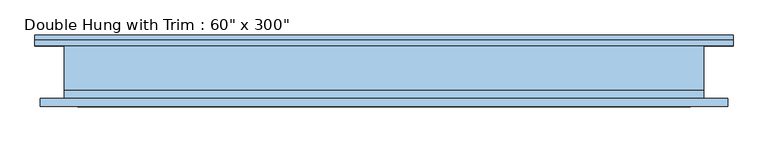
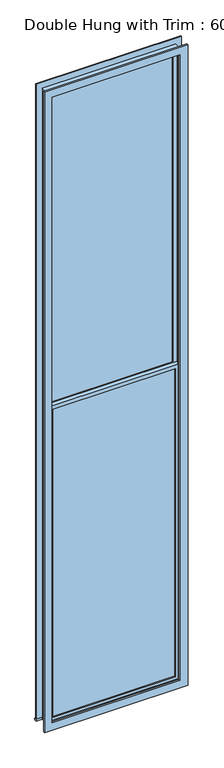
"""IFC4 building model written with IfcOpenShell, lengths in millimetres: window geometry."""

from ifc_helpers import new_model, si_unit, frame, origin, place, context, project, spatial, polyline, outline, extrude, source, transform, mapped, element, save


def window_120b3672(model_context):
    return source(origin(), model_context, "Body", "SweptSolid", [
        extrude(outline(polyline([(-698.5, -15.875), (698.5, -15.875), (698.5, -28.575), (-698.5, -28.575), (-698.5, -15.875)])), frame((0.0, 0.0, 977.9), z_axis=(0.0, 0.0, 1.0), x_axis=(1.0, 0.0, 0.0)), (0.0, 0.0, 1.0), 3724.275),
        extrude(outline(polyline([(4746.625, -742.95), (933.45, -742.95), (933.45, 742.95), (4746.625, 742.95), (4746.625, -742.95)]), holes=[polyline([(4702.175, -698.5), (4702.175, 698.5), (977.9, 698.5), (977.9, -698.5), (4702.175, -698.5)])]), frame((0.0, -44.45, 0.0), z_axis=(0.0, 1.0, 0.0), x_axis=(0.0, 0.0, 1.0)), (0.0, 0.0, 1.0), 44.45),
        extrude(outline(polyline([(-831.85, 88.9), (831.85, 88.9), (831.85, 63.5), (-831.85, 63.5), (-831.85, 88.9)])), frame((0.0, 0.0, 914.4), z_axis=(0.0, 0.0, 1.0), x_axis=(1.0, 0.0, 0.0)), (0.0, 0.0, 1.0), 19.05),
        extrude(outline(polyline([(8515.35, -742.95), (8515.35, 742.95), (933.45, 742.95), (933.45, 831.85), (8604.25, 831.85), (8604.25, -831.85), (933.45, -831.85), (933.45, -742.95), (8515.35, -742.95)])), frame((0.0, 63.5, 0.0), z_axis=(0.0, 1.0, 0.0), x_axis=(0.0, 0.0, 1.0)), (0.0, 0.0, 1.0), 12.7),
        extrude(outline(polyline([(8591.55, 819.15), (8591.55, -819.15), (857.25, -819.15), (857.25, 819.15), (8591.55, 819.15)]), holes=[polyline([(8502.65, 730.25), (946.15, 730.25), (946.15, -730.25), (8502.65, -730.25), (8502.65, 730.25)])]), frame((0.0, -82.55, 0.0), z_axis=(0.0, 1.0, 0.0), x_axis=(0.0, 0.0, 1.0)), (0.0, 0.0, 1.0), 19.05),
        extrude(outline(polyline([(698.5, 15.875), (-698.5, 15.875), (-698.5, 28.575), (698.5, 28.575), (698.5, 15.875)])), frame((0.0, 0.0, 4746.625), z_axis=(0.0, 0.0, 1.0), x_axis=(1.0, 0.0, 0.0)), (0.0, 0.0, 1.0), 3724.275),
        extrude(outline(polyline([(8515.35, -742.95), (4702.175, -742.95), (4702.175, 742.95), (8515.35, 742.95), (8515.35, -742.95)]), holes=[polyline([(8470.9, -698.5), (8470.9, 698.5), (4746.625, 698.5), (4746.625, -698.5), (8470.9, -698.5)])]), frame((0.0, 0.0, 0.0), z_axis=(0.0, 1.0, 0.0), x_axis=(0.0, 0.0, 1.0)), (0.0, 0.0, 1.0), 44.45),
        extrude(outline(polyline([(8534.4, -762.0), (914.4, -762.0), (914.4, 762.0), (8534.4, 762.0), (8534.4, -762.0)]), holes=[polyline([(8502.65, -730.25), (8502.65, 730.25), (946.15, 730.25), (946.15, -730.25), (8502.65, -730.25)])]), frame((0.0, -63.5, 0.0), z_axis=(0.0, 1.0, 0.0), x_axis=(0.0, 0.0, 1.0)), (0.0, 0.0, 1.0), 19.05),
        extrude(outline(polyline([(8534.4, 762.0), (8534.4, -762.0), (914.4, -762.0), (914.4, 762.0), (8534.4, 762.0)]), holes=[polyline([(8515.35, 742.95), (933.45, 742.95), (933.45, -742.95), (8515.35, -742.95), (8515.35, 742.95)])]), frame((0.0, -44.45, 0.0), z_axis=(0.0, 1.0, 0.0), x_axis=(0.0, 0.0, 1.0)), (0.0, 0.0, 1.0), 107.95),
    ])


if __name__ == "__main__":
    model = new_model("IFC4")
    model_context = context("Model", 3, world=origin())
    ifc_project = project(units=[si_unit("LENGTHUNIT", "METRE", prefix="MILLI")], contexts=[model_context])
    site = spatial("IfcSite", under=ifc_project)
    building = spatial("IfcBuilding", under=site)
    placement = place(None, origin())
    window_shape = window_120b3672(model_context)
    element("IfcWindow", 1, ObjectType="Double Hung with Trim : 60\" x 300\"", at=placement, inside=building, context=model_context, shape_type="MappedRepresentation", body=[
        mapped(window_shape, transform((0.0, 0.0, 0.0), x_axis=(1.0, 0.0, 0.0), y_axis=(0.0, 1.0, 0.0), z_axis=(0.0, 0.0, 1.0))),
    ])
    save(model, "model.ifc")

# Revit data of these elements
# Type "Double Hung with Trim : 60\" x 300\""
#   Type Mark = "28"
#   Construction Type Id = "GSP4R"
#   Assembly Code = "B2020100"
#   Analytic Construction = "1/8 in Pilkington single glazing"
#   Visual Light Transmittance = 0.9
#   Solar Heat Gain Coefficient = 0.78
#   Heat Transfer Coefficient (U) = 0.6496 BTU/(h·ft²·°F)
#   Height = 25' - 0"
#   Default Sill Height = 3' - 0"
#   Trim Projection - Ext. = 0' - 0 1/2"
#   Trim Projection - Int. = 0' - 0 3/4"
#   Trim Width - Exterior = 0' - 3 1/2"
#   Trim Width - Interior = 0' - 3 1/2"
#   Width = 5' - 0"
#   Window Inset = 0' - 0 3/4"
#   Define Thermal Properties by = 1
#   Glass Pane Material = Glass
#   Sash Material = Sash
#   Trim Exterior Material = Trim
#   Trim Interior Material = Trim
#   Wall Closure = (empty or 0)
# Element 1 (IfcWindow, "Double Hung with Trim : 60\" x 300\"")
#   Materials on its faces: "Sash", "Trim", "Glass"
# Materials
#   "Glass": class "Glass", colour RGB 0 128 192, transparency 0.75, Description = "Soda Lime Glass", Cost = 0
#   "Sash": class "Wood", colour RGB 224 178 126, transparency 0
#   "Trim": class "Wood", colour RGB 224 178 126, transparency 0
